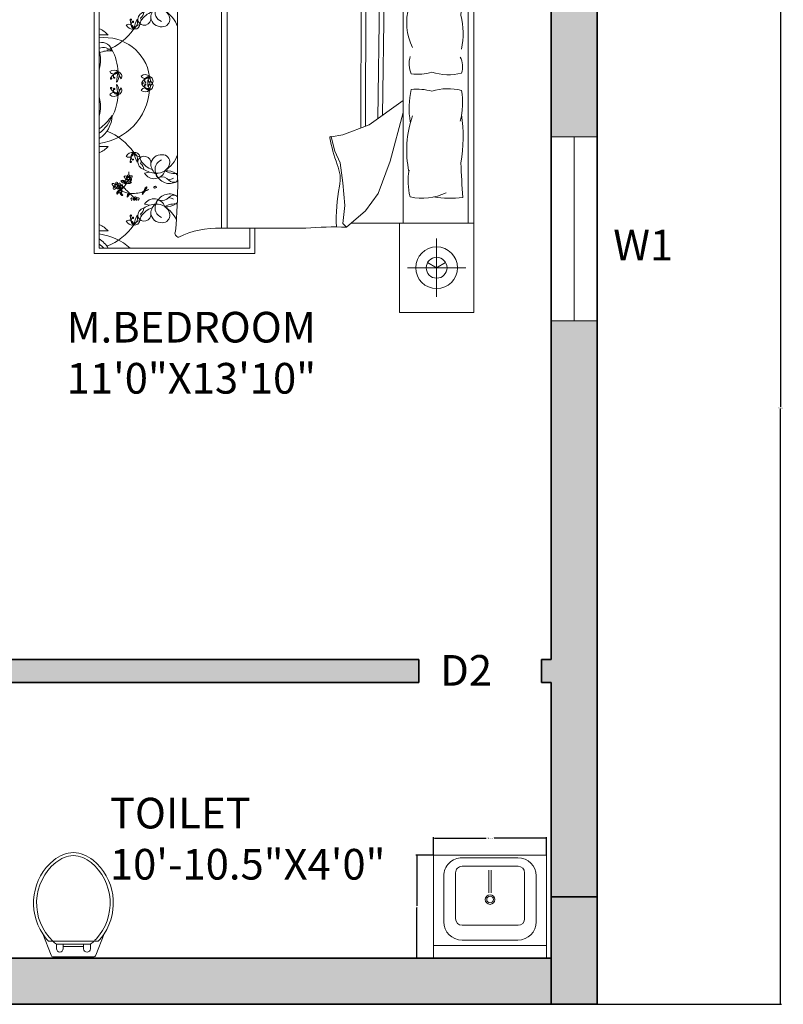
# Model space of a CAD drawing. Units: inches. Extents: x -9 to 505, y -680 to 48.
# Tile 5 of 17: x 356 to 505, y -680 to -487. Entities that reach past the tile are written whole.
import ezdxf

# ---------------------------------------------------------------- set-up
doc = ezdxf.new("R2010")
doc.units = ezdxf.units.IN
doc.header["$MEASUREMENT"] = 0
for name, color, linetype, lineweight in [('A-ANNO-DIMS', 2, 'Continuous', 18), ('A-ANNO-TEXT', 7, 'Continuous', 18), ('A-AREA-IDEN', 7, 'Continuous', 18), ('A-FLOR-FIXT', 9, 'Continuous', 18), ('A-FURN', 8, 'Continuous', 18), ('A-GLAZ', 4, 'Continuous', 18), ('A-WALL', 7, 'Continuous', 35), ('A-WALL-PATT', 251, 'Continuous', 13), ('S-CONC', 7, 'Continuous', 35), ('S-CONC-PATT', 18, 'Continuous', 13), ('WC-Detail_dwgmodels.com', 251, 'Continuous', 13), ('WC-Outline_dwgmodels.com', 250, 'Continuous', 18)]:
    doc.layers.add(name, color=color, linetype=linetype, lineweight=lineweight)
doc.styles.get("Standard").update_dxf_attribs({"font": 'arial.ttf'})
doc.dimstyles.get("Standard").update_dxf_attribs({"dimtxt": 0.18, "dimasz": 0.18, "dimexe": 0.18, "dimexo": 0.0625, "dimgap": 0.09, "dimtad": 0, "dimtih": 1, "dimtoh": 1, "dimdec": 0, "dimzin": 0, "dimdsep": 46, "dimlunit": 3, "dimtxsty": 'Standard', "dimcen": 0.09, "dimadec": 0, "dimazin": 0, "dimtfac": 1, "dimtdec": 0, "dimtofl": 0, "dimtmove": 0, "dimatfit": 3, "dimfxl": 1, "dimtolj": 1, "dimtzin": 0, "dimarcsym": 0})

# ---------------------------------------------------------------- blocks, each defined once
blk = doc.blocks.new('М14 600х655')
for p, q in [((-655, 600), (-655, 0)), ((-655, 600), (-655, 0)), ((-655, 0), (-655, 600)), ((0, 600), (-655, 600)), ((0, 0), (0, 600)), ((0, 525), (-655, 525)), ((-165.1, 494.1), (-489.9, 494.1)), ((-165.4, 408.4), (-490.2, 408.4)), ((-595.8, 388.1), (-595.8, 121.3)), ((-528.4, 370.1), (-528.4, 103.3)), ((-127.2, 103.3), (-127.2, 370.1)), ((-59.2, 121.3), (-59.2, 388.1)), ((-333.5, 87.1), (-333.5, 219.6)), ((-321.5, 87.1), (-321.5, 219.6)), ((-490.2, 65.1), (-165.4, 65.1)), ((-655, 0), (-655, 0)), ((-655, 0), (-655, 0)), ((-655, 0), (0, 0)), ((-655, 0), (0, 0)), ((-489.9, 15.4), (-165.1, 15.4))]:
    blk.add_line(p, q)
for radius in [27.6, 19.3]:
    blk.add_circle((-327.5, 258.9), radius)
for centre, radius, start, end in [((-489.9, 388.1), 105.9, 90, 180), ((-165.1, 388.1), 105.9, 0, 90), ((-490.2, 370.1), 38.2, 90, 180), ((-165.4, 370.1), 38.2, 0, 90), ((-489.9, 121.3), 105.9, 180, 270), ((-165.1, 121.3), 105.9, 270, 0), ((-490.2, 103.3), 38.2, 180, 270), ((-165.4, 103.3), 38.2, 270, 0)]:
    blk.add_arc(centre, radius, start, end)
blk = doc.blocks.new('BED-DOUBLE-WITH-NIGHTSTANDS')
for p, q in [((74.3, 0), (74.3, 87.37)), ((67.02, 72.93), (67.02, 84.34)), ((61.31, 78.63), (72.73, 78.63)), ((0, 75.23), (0, 11.53)), ((31.47, 75.23), (0, 75.23)), ((31.47, 70.38), (31.47, 75.23)), ((1.01, 74.22), (30.46, 74.22)), ((1.01, 12.54), (1.01, 74.22)), ((30.46, 74.22), (30.46, 70.37)), ((24.93, 70.38), (24.93, 16.47)), ((26.02, 70.29), (26.02, 16.47)), ((52.32, 69.59), (52.18, 36.06)), ((53.22, 69.58), (53.09, 36.41)), ((55.97, 69.63), (55.52, 37.9)), ((56.87, 69.66), (56.43, 38.56)), ((60.5, 17.47), (60.5, 69.9)), ((73.18, 69.9), (73.18, 17.47)), ((9.87, 65.61), (10.86, 65.8)), ((16.35, 61.42), (16.35, 25.95)), ((9.87, 59.5), (10.86, 59.31)), ((60.5, 41.48), (53.83, 36.69)), ((57.9, 29.61), (60.5, 39.14)), ((53.83, 36.69), (48.7, 34.74)), ((48.7, 34.74), (46.4, 34.39)), ((46.4, 34.39), (47.11, 31.56)), ((47.11, 31.56), (48.17, 29.26)), ((48.17, 29.26), (48.7, 25.36)), ((55.6, 23.24), (57.9, 29.61)), ((9.87, 27.26), (10.86, 27.45)), ((48.7, 25.36), (49.06, 20.94)), ((53.12, 19.88), (55.6, 23.24)), ((9.87, 21.15), (10.86, 20.96)), ((49.06, 20.94), (48.7, 17.4)), ((49.41, 16.69), (53.12, 19.88)), ((48.7, 17.4), (49.41, 16.69)), ((74.3, 17.47), (50.32, 17.47)), ((30.46, 16.47), (30.46, 12.54)), ((31.47, 11.53), (31.47, 16.47)), ((67.02, 14.45), (67.02, 3.03)), ((30.46, 12.54), (1.01, 12.54)), ((0, 11.53), (31.47, 11.53)), ((61.31, 8.74), (72.73, 8.74))]:
    blk.add_line(p, q)
for points in [[(74.3, 69.9), (59.74, 69.9), (59.74, 87.37), (74.3, 87.37)], [(67.02, 78.63), (65.26, 77.62)], [(67.02, 78.63), (68.79, 77.62)], [(59.74, 17.47), (59.74, 0), (74.3, 0)], [(67.02, 8.74), (65.26, 9.76)], [(67.02, 8.74), (68.79, 9.76)]]:
    blk.add_lwpolyline(points)
for points in [[(26.71, 70.27, -0.056112), (21.91, 70.9, -0.095341), (17.28, 72.13)], [(72.13, 64.88, 0.074897), (66.42, 64.77, -0.472817)], [(66.1, 47.01, 0.14099), (71.92, 46.83, 0.235245)], [(66.1, 43.28, -0.14099), (71.92, 43.45, -0.235245)], [(72.13, 22.49, -0.074897), (66.42, 22.6, 0.472817)], [(41.41, 16.51, -0.001242), (24.83, 16.47, 0.127202), (16.57, 14.72)]]:
    blk.add_lwpolyline(points, format="xyb")
for centre, radius in [((67.02, 78.63), 4.08), ((67.02, 78.63), 2.04), ((4.36, 62.02), 0.223), ((6.7, 60.56), 0.223), ((6.7, 26.2), 0.223), ((4.36, 24.75), 0.223), ((67.02, 8.74), 4.08), ((67.02, 8.74), 2.04)]:
    blk.add_circle(centre, radius)
for centre, radius, start, end in [((-2.05, 76.99), 5.56, 303.4617, 330.1116), ((-3.09, 78.99), 6.93, 306.3036, 316.4814), ((-0.53, 82.71), 11.41, 277.745, 311.8856), ((-1.65, 63.19), 11.41, 34.3865, 68.5908), ((16.83, 71.47), 0.796, 56.1736, 203.4781), ((-0.77, 73.87), 4.64, 292.5547, 318.9546), ((1.73, 86.58), 15.79, 267.4081, 273.6519), ((7.49, 68.4), 1.27, 77.7115, 159.0387), ((6.81, 69.66), 0.953, 238.4633, 358.2869), ((9.93, 67.74), 2.89, 138.8402, 177.9352), ((8.2, 68.81), 0.933, 117.6827, 223.7762), ((7.99, 68.72), 0.946, 2.9516, 103.728), ((15.55, 71.37), 7.98, 192.5173, 207.1824), ((6.71, 68.17), 1.8, 345.4653, 54.2343), ((9.43, 70.65), 1.95, 211.3827, 255.2969), ((-68.63, 64.1), 85.02, 358.1965, 4.7598), ((44.11, 274.32), 204.79, 265.1265, 270.8855), ((49.82, 226.53), 156.99, 269.0718, 273.9), ((7.19, 67.84), 0.142, 177.9352, 11.4834), ((7.26, 67.85), 0.0688, 11.4834, 127.9409), ((7.66, 68.26), 0.0744, 223.7729, 159.7333), ((9.8, 67.61), 1.31, 350.264, 160.8688), ((10.19, 67.92), 1.64, 175.969, 254.3045), ((8.38, 67.88), 0.804, 333.9755, 53.2681), ((8.02, 66.16), 1.74, 6.1662, 51.5825), ((12.69, 70.21), 4.12, 211.2614, 251.7045), ((13.16, 67.13), 2.09, 84.9449, 172.8857), ((13.96, 66.31), 2.03, 111.5819, 201.4221), ((12.28, 68.18), 2.63, 265.2933, 346.921), ((13.37, 67.73), 1.48, 354.4856, 91.0538), ((10.2, 71.58), 6.61, 303.6671, 336.3547), ((12.35, 70.24), 4.69, 236.2883, 266.5076), ((11.75, 66.69), 2.17, 209.9085, 343.1337), ((13.63, 67.49), 2.54, 182.3591, 234.0401), ((14.13, 62.72), 3.37, 122.7011, 126.3445), ((15.71, 69.16), 3.62, 238.8218, 280.751), ((14.13, 62.72), 3.37, 55.785, 94.7304), ((4.68, 63.45), 0.248, 124.3538, 214.3923), ((5.21, 63.62), 0.673, 176.9701, 248.2913), ((10.01, 67.17), 6.5, 212.6784, 216.3746), ((5.6, 63.28), 0.579, 122.8155, 187.3992), ((5.86, 63.21), 0.673, 109.4799, 177.6828), ((5.5, 63.63), 0.248, 56.8636, 146.9021), ((10.97, 60.13), 6.5, 145.1882, 148.8844), ((8.96, 64.13), 2.46, 178.3264, 187.1302), ((6.3, 63.79), 0.459, 11.3256, 64.4621), ((7.86, 64.45), 1.38, 190.2588, 210.656), ((6.93, 63.89), 0.419, 188.3432, 274.2869), ((7.3, 64.12), 0.732, 210.656, 242.6341), ((7.85, 64.75), 1.4, 218.2101, 226.3071), ((6.82, 63.57), 0.178, 325.7657, 67.4417), ((1.29, 69.52), 8.3, 313.1541, 322.0459), ((7.39, 64.54), 0.171, 142.4737, 265.053), ((7.61, 64.57), 0.367, 127.7621, 169.0403), ((7.42, 64.88), 0.517, 265.053, 338.3618), ((8.1, 64.17), 0.676, 113.4276, 137.6104), ((8.03, 64.87), 0.223, 183.2768, 356.7232), ((8.19, 64.47), 0.364, 139.7889, 227.6792), ((8.07, 64.34), 0.192, 227.6792, 350.3487), ((7.33, 64.48), 0.728, 353.0852, 15.7171), ((7.81, 64.39), 0.46, 350.3487, 43.6538), ((8.66, 64.86), 0.535, 198.7263, 262.5032), ((8.24, 64.61), 0.213, 1.1081, 91.8675), ((8.64, 64.5), 0.172, 255.2356, 54.9248), ((8.37, 64.57), 0.371, 11.5637, 52.6358), ((11.9, 63.61), 2.46, 178.3264, 187.1302), ((9.24, 63.27), 0.459, 11.3256, 64.4621), ((10.8, 63.93), 1.38, 190.2588, 210.656), ((12.67, 65.32), 0.542, 167.3041, 285.1471), ((14.77, 66.35), 2.78, 199.2822, 299.1751), ((13.28, 63.06), 1.79, 41.5653, 105.1471), ((14.26, 66.77), 2.51, 277.436, 299.9149), ((15.59, 65.12), 1.31, 221.5653, 293.8354), ((15.39, 64.67), 1.05, 17.4186, 52.325), ((15.39, 64.67), 1.05, 314.4517, 343.3657), ((73.15, 61.76), 11.71, 165.1039, 191.0369), ((64.13, 53.75), 11.26, 65.1316, 101.7583), ((903.62, 16.72), 832.89, 176.68521, 177.14978), ((3.72, 61.68), 0.171, 142.4737, 265.053), ((3.95, 61.71), 0.367, 61.2196, 169.0403), ((3.75, 62.02), 0.517, 265.053, 338.3618), ((4.19, 62.47), 0.439, 157.4086, 261.4386), ((3.94, 62.48), 0.22, 58.0499, 135.6268), ((4.44, 61.32), 0.676, 113.4276, 137.6104), ((4.17, 62.34), 0.147, 172.906, 277.132), ((3.69, 62.07), 0.702, 14.7558, 58.0499), ((4.52, 61.61), 0.364, 139.7889, 227.6792), ((4.67, 62.26), 0.303, 36.1046, 181.4281), ((3.66, 61.62), 0.728, 353.0852, 15.7171), ((4.14, 61.53), 0.46, 350.3487, 43.6538), ((5.05, 63.41), 0.579, 190.3057, 287.1958), ((4.49, 62.5), 0.306, 270.0645, 331.1507), ((4.75, 62.43), 0.35, 221.8413, 265.7877), ((4.99, 62.01), 0.535, 198.7263, 262.5032), ((4.57, 61.76), 0.213, 1.1081, 91.8675), ((4.75, 62.29), 0.218, 263.7526, 41.7054), ((4.7, 61.71), 0.371, 11.5637, 86.365), ((4.99, 63.46), 0.257, 216.3746, 291.7548), ((7.26, 59.85), 3.63, 124.0033, 132.4917), ((4.97, 61.64), 0.172, 255.2356, 54.9248), ((3.53, 59.39), 3.88, 63.7819, 68.2913), ((5.6, 62.38), 0.616, 128.3208, 208.8162), ((5.71, 62.42), 0.737, 207.7043, 254.3516), ((5.16, 63.04), 0.194, 289.3605, 111.7548), ((5.3, 63.04), 0.194, 221.8703, 44.2646), ((6.18, 62.48), 1.01, 157.2305, 229.0635), ((5.84, 62.81), 0.597, 174.4544, 220.6188), ((5.23, 62), 1.01, 270.278, 342.111), ((2.45, 59.48), 4.35, 30.544, 49.818), ((5.62, 63.36), 0.257, 148.8844, 224.2646), ((4.84, 61.96), 0.717, 340.0041, 40.6188), ((7.26, 59.85), 3.63, 94.756, 119.2041), ((14.99, 54.63), 11.94, 132.2412, 142.1744), ((5.71, 62.03), 0.597, 278.7227, 324.8872), ((6.81, 61.72), 0.616, 182.8499, 266.1226), ((6.57, 62.16), 0.597, 231.7607, 277.9252), ((7.04, 62.26), 1.01, 214.5369, 286.3699), ((7.45, 56.25), 7.24, 73.5842, 93.8277), ((9.87, 63.37), 0.419, 188.3432, 274.2869), ((10.24, 63.6), 0.732, 210.656, 242.6341), ((10.79, 64.23), 1.4, 218.2101, 226.3071), ((9.76, 63.05), 0.178, 325.7657, 67.4417), ((10.26, 62.72), 0.419, 147.5332, 233.4768), ((10.63, 62.94), 0.732, 179.1859, 211.164), ((9.92, 62.77), 0.178, 354.3784, 96.0543), ((7.45, 56.25), 7.24, 63.0032, 69.8941), ((11.19, 63.27), 1.38, 211.164, 231.5612), ((11.43, 64.4), 2.46, 234.6898, 243.4936), ((11.45, 63.13), 1.4, 195.5129, 203.6099), ((9.87, 62.21), 0.459, 357.3579, 50.4944), ((11.84, 62.3), 0.168, 12.7051, 190.4384), ((11.95, 62.32), 0.274, 190.4384, 10.4136), ((4.41, 61.49), 0.192, 227.6792, 350.3487), ((5.91, 60.73), 0.717, 98.7227, 159.3375), ((5.55, 61.65), 0.737, 244.9899, 291.6373), ((5.61, 61.55), 0.616, 290.5253, 358.5375), ((6.07, 60.22), 0.171, 142.4737, 265.053), ((6.29, 60.26), 0.367, 61.2196, 169.0403), ((6.1, 60.57), 0.517, 265.053, 338.3618), ((6.53, 61.01), 0.439, 157.4086, 261.4386), ((6.29, 61.03), 0.22, 58.0499, 135.6268), ((6.78, 59.86), 0.676, 113.4276, 137.6104), ((6.52, 60.89), 0.147, 172.906, 277.132), ((6.03, 60.62), 0.702, 14.7558, 58.0499), ((2.45, 59.48), 4.35, 23.0501, 23.8477), ((6.87, 60.16), 0.364, 139.7889, 227.6792), ((6.75, 60.03), 0.192, 227.6792, 350.3487), ((6.75, 60.86), 0.717, 37.3105, 97.9252), ((7.01, 60.81), 0.303, 36.1046, 181.4281), ((6.01, 60.16), 0.728, 353.0852, 15.7171), ((6.83, 61.84), 0.737, 265.0106, 311.658), ((2.45, 59.48), 4.35, 357.1071, 4.7585), ((6.49, 60.07), 0.46, 350.3487, 43.6538), ((7.34, 60.55), 0.535, 198.7263, 262.5032), ((6.84, 61.04), 0.306, 270.0645, 331.1507), ((7.1, 60.97), 0.35, 221.8413, 265.7877), ((6.91, 60.3), 0.213, 1.1081, 91.8675), ((7.1, 60.84), 0.218, 263.7526, 41.7054), ((7.05, 60.25), 0.371, 11.5637, 86.365), ((7.31, 60.19), 0.172, 255.2356, 54.9248), ((11.75, 58.42), 2.17, 16.8663, 150.0915), ((12.67, 59.79), 0.542, 74.8529, 192.6959), ((14.77, 58.76), 2.78, 60.8249, 160.7178), ((13.28, 62.05), 1.79, 254.8529, 318.4347), ((14.26, 58.33), 2.51, 60.0851, 82.564), ((15.59, 59.99), 1.31, 66.1646, 138.4347), ((15.39, 60.44), 1.05, 307.675, 336.7144), ((15.39, 60.44), 1.05, 23.2856, 45.5483), ((72.29, 56.71), 11.12, 163.8254, 206.1239), ((10.19, 57.19), 1.64, 105.6955, 184.031), ((8.02, 58.95), 1.74, 308.4175, 353.8338), ((12.69, 54.9), 4.12, 108.2955, 148.7386), ((12.35, 54.86), 4.69, 93.4924, 123.7117), ((13.63, 57.62), 2.54, 125.9599, 177.6409), ((13.96, 58.8), 2.03, 158.5779, 248.4181), ((12.28, 56.93), 2.63, 13.079, 94.7067), ((14.13, 62.39), 3.37, 233.6555, 237.2989), ((15.71, 55.95), 3.62, 79.7133, 121.1782), ((14.13, 62.39), 3.37, 265.2696, 304.215), ((10.2, 53.53), 6.61, 21.4941, 56.3329), ((56.84, 54.51), 15.36, 348.8159, 13.6573), ((6.81, 55.44), 0.953, 1.7131, 121.5367), ((7.49, 56.71), 1.27, 200.9613, 282.2885), ((7.19, 57.27), 0.142, 348.5166, 182.0648), ((9.93, 57.37), 2.89, 182.0648, 221.1598), ((7.26, 57.26), 0.0688, 232.0591, 348.5166), ((8.2, 56.3), 0.933, 136.2238, 242.3173), ((7.61, 56.86), 0.123, 200.2817, 136.2238), ((6.71, 56.94), 1.8, 305.7657, 14.5347), ((15.55, 53.74), 7.98, 152.8176, 167.4827), ((7.99, 56.39), 0.946, 256.272, 357.0484), ((9.43, 54.46), 1.95, 104.7031, 148.6173), ((9.8, 57.5), 1.31, 199.1312, 9.736), ((8.38, 57.23), 0.804, 306.7319, 26.0245), ((13.16, 57.98), 2.09, 187.1143, 275.0551), ((13.37, 57.38), 1.48, 268.9462, 5.5144), ((-0.77, 51.23), 4.64, 41.0454, 67.4453), ((1.73, 38.53), 15.79, 86.3481, 92.5919), ((-1.65, 61.92), 11.41, 291.4092, 325.6135), ((2.11, 44.94), 8.83, 8.1803, 97.1364), ((1.49, 50.77), 2.05, 10.9261, 103.6102), ((1.78, 49.23), 2.59, 48.0951, 107.1391), ((-4.99, 49.37), 6.27, 343.5431, 17.0202), ((2.92, 46.08), 5.11, 83.3805, 111.883), ((-6.64, 46.18), 11.41, 4.4623, 27.4146), ((66.26, 48.62), 4.63, 161.4593, 204.9817), ((67.77, 48.03), 4.32, 343.8974, 26.6563), ((-8.22, 46.89), 9.28, 4.3787, 5.6357), ((-14.58, 42), 16.58, 19.7217, 19.9028), ((3.89, 46.13), 1.27, 47.7873, 129.1145), ((3.93, 47.57), 0.953, 208.5391, 328.3627), ((5.67, 44.34), 2.89, 108.9159, 148.011), ((4.7, 46.14), 0.933, 87.7585, 193.852), ((12.35, 44.68), 7.98, 162.593, 177.2582), ((3.09, 46.33), 1.8, 315.5411, 24.3101), ((6.69, 47.12), 1.95, 181.4585, 225.3727), ((4.47, 46.16), 0.946, 333.0274, 73.8037), ((10, 45.26), 1.27, 47.7873, 129.1145), ((63.18, 57.31), 10.71, 264.0129, 285.8293), ((3.35, 45.79), 0.142, 148.011, 341.5592), ((3.42, 45.77), 0.0688, 341.5592, 98.0167), ((3.96, 45.93), 0.0744, 193.9791, 129.8091), ((12.35, 44.99), 7.98, 182.7418, 197.407), ((3.09, 43.35), 1.8, 335.6899, 44.4589), ((10.04, 46.7), 0.953, 208.5391, 328.3627), ((9.46, 44.92), 0.142, 148.011, 341.5592), ((9.46, 44.75), 0.142, 18.4408, 211.989), ((11.79, 43.47), 2.89, 108.9159, 148.011), ((11.79, 46.21), 2.89, 211.989, 251.0841), ((9.53, 44.9), 0.0688, 341.5592, 98.0167), ((9.53, 44.78), 0.0688, 261.9833, 18.4408), ((10.81, 45.26), 0.933, 87.7585, 193.852), ((10.81, 44.41), 0.933, 166.148, 272.2415), ((10.03, 44.6), 0.123, 230.0755, 166.148), ((10.07, 45.06), 0.0744, 193.9791, 129.8091), ((9.21, 45.45), 1.8, 315.5411, 24.3101), ((18.47, 43.81), 7.98, 162.593, 177.2582), ((9.21, 44.22), 1.8, 335.6899, 44.4589), ((18.47, 45.87), 7.98, 182.7418, 197.407), ((10.59, 45.29), 0.946, 333.0274, 73.8037), ((12.8, 46.25), 1.95, 181.4585, 225.3727), ((10.59, 44.39), 0.946, 286.1963, 26.9726), ((12.8, 43.43), 1.95, 134.6273, 178.5415), ((-0.53, 44.37), 11.41, 277.745, 355.5377), ((3.93, 42.1), 0.953, 31.6373, 151.4609), ((3.89, 43.54), 1.27, 230.8855, 312.2127), ((3.35, 43.88), 0.142, 18.4408, 211.989), ((5.67, 45.33), 2.89, 211.989, 251.0841), ((3.42, 43.9), 0.0688, 261.9833, 18.4408), ((-6.64, 43.49), 11.41, 332.5854, 355.5377), ((4.7, 43.54), 0.933, 166.148, 272.2415), ((3.92, 43.73), 0.123, 230.0755, 166.148), ((6.69, 42.55), 1.95, 134.6273, 178.5415), ((4.47, 43.51), 0.946, 286.1963, 26.9726), ((10.04, 42.98), 0.953, 31.6373, 151.4609), ((10, 44.41), 1.27, 230.8855, 312.2127), ((77.04, 40), 15.41, 166.3762, 190.1383), ((63.18, 32.98), 10.71, 74.1707, 95.9871), ((56.52, 41.16), 15.57, 346.04, 8.4751), ((-4.99, 40.3), 6.27, 342.9798, 16.4569), ((-8.22, 42.79), 9.28, 354.3643, 355.6213), ((-14.58, 47.67), 16.58, 340.0972, 340.2783), ((40.51, 34.46), 31.69, 350.503, 7.7804), ((-2.05, 38.64), 5.56, 303.4617, 358.728), ((-5.04, 44.28), 10.31, 305.947, 325.9877), ((-3.09, 40.64), 6.93, 306.3036, 342.1496), ((81.47, 31.77), 20.31, 160.7385, 191.9603), ((-1.65, 24.85), 11.41, 34.3865, 68.5908), ((46.33, 34.19), 0.211, 70.2464, 181.1377), ((79.42, 40.46), 33.88, 190.6617, 199.8806), ((1.73, 48.24), 15.79, 267.4081, 273.6519), ((-0.77, 35.53), 4.64, 292.5547, 318.9546), ((7.49, 30.05), 1.27, 77.7115, 159.0387), ((6.81, 31.32), 0.953, 238.4633, 358.2869), ((9.93, 29.39), 2.89, 138.8402, 177.9352), ((8.2, 30.46), 0.933, 117.6827, 223.7762), ((7.99, 30.37), 0.946, 2.9516, 103.728), ((9.43, 32.3), 1.95, 211.3827, 255.2969), ((6.71, 29.83), 1.8, 345.4653, 54.2343), ((15.55, 33.02), 7.98, 192.5173, 207.1824), ((13.16, 28.78), 2.09, 84.9449, 172.8857), ((13.37, 29.38), 1.48, 354.4856, 91.0538), ((7.19, 29.49), 0.142, 177.9352, 11.4834), ((7.26, 29.5), 0.0688, 11.4834, 127.9409), ((7.66, 29.92), 0.0744, 223.7729, 159.7333), ((9.8, 29.26), 1.31, 350.264, 160.8688), ((10.19, 29.57), 1.64, 175.969, 254.3045), ((8.38, 29.53), 0.804, 333.9755, 53.2681), ((8.02, 27.81), 1.74, 6.1662, 51.5825), ((12.69, 31.86), 4.12, 211.2614, 251.7045), ((13.63, 29.14), 2.54, 182.3591, 234.0401), ((13.96, 27.96), 2.03, 111.5819, 201.4221), ((12.28, 29.84), 2.63, 265.2933, 346.921), ((10.2, 33.24), 6.61, 303.6671, 338.5059), ((41.05, 26.07), 7.11, 348.6608, 23.7384), ((903.62, 70.65), 832.89, 182.85022, 183.31479), ((2.45, 27.28), 4.35, 355.2415, 2.8929), ((12.35, 31.9), 4.69, 236.2883, 266.5076), ((11.75, 28.34), 2.17, 209.9085, 343.1337), ((12.67, 26.97), 0.542, 167.3041, 285.1471), ((14.13, 24.37), 3.37, 122.7011, 126.3445), ((14.77, 28.01), 2.78, 199.2822, 299.1751), ((15.71, 30.81), 3.62, 238.8218, 280.2867), ((14.13, 24.37), 3.37, 55.785, 94.7304), ((15.39, 26.33), 1.05, 23.2856, 52.325), ((73.15, 25.61), 11.71, 168.9631, 194.8961), ((3.72, 25.08), 0.171, 94.947, 217.5263), ((3.75, 24.74), 0.517, 21.6382, 94.947), ((4.52, 25.15), 0.364, 132.3208, 220.2111), ((4.41, 25.28), 0.192, 9.6513, 132.3208), ((3.66, 25.14), 0.728, 344.2829, 6.9148), ((4.14, 25.23), 0.46, 316.3462, 9.6513), ((4.99, 24.76), 0.535, 97.4968, 161.2737), ((4.97, 25.12), 0.172, 305.0752, 104.7644), ((5.71, 24.34), 0.737, 105.6484, 152.2957), ((6.18, 24.28), 1.01, 130.9365, 202.7695), ((5.55, 25.11), 0.737, 68.3627, 115.0101), ((5.23, 24.76), 1.01, 17.889, 89.722), ((5.91, 26.03), 0.717, 200.6625, 261.2773), ((2.45, 27.28), 4.35, 310.182, 329.456), ((4.84, 24.8), 0.717, 319.3812, 19.9959), ((5.71, 24.73), 0.597, 35.1128, 81.2773), ((5.61, 25.22), 0.616, 1.4625, 69.4747), ((6.07, 26.54), 0.171, 94.947, 217.5263), ((6.29, 26.51), 0.367, 190.9597, 298.7804), ((6.1, 26.19), 0.517, 21.6382, 94.947), ((6.53, 25.75), 0.439, 98.5614, 202.5914), ((6.29, 25.74), 0.22, 224.3732, 301.9501), ((6.81, 25.04), 0.616, 93.8774, 177.1501), ((7.04, 24.5), 1.01, 73.6301, 145.4631), ((6.57, 24.61), 0.597, 82.0748, 128.2393), ((6.78, 26.9), 0.676, 222.3896, 246.5724), ((6.52, 25.87), 0.147, 82.868, 187.094), ((6.03, 26.14), 0.702, 301.9501, 345.2442), ((2.45, 27.28), 4.35, 336.1523, 336.9499), ((6.87, 26.61), 0.364, 132.3208, 220.2111), ((6.75, 26.73), 0.192, 9.6513, 132.3208), ((6.75, 25.91), 0.717, 262.0748, 322.6895), ((6.01, 26.6), 0.728, 344.2829, 6.9148), ((7.01, 25.96), 0.303, 178.5719, 323.8954), ((6.83, 24.92), 0.737, 48.342, 94.9894), ((6.49, 26.69), 0.46, 316.3462, 9.6513), ((7.34, 26.21), 0.535, 97.4968, 161.2737), ((7.1, 25.79), 0.35, 94.2123, 138.1587), ((6.84, 25.72), 0.306, 28.8493, 89.9355), ((6.91, 26.46), 0.213, 268.1325, 358.8919), ((7.05, 26.51), 0.371, 273.635, 348.4363), ((7.1, 25.92), 0.218, 318.2946, 96.2474), ((7.31, 26.58), 0.172, 305.0752, 104.7644), ((13.28, 24.72), 1.79, 41.5653, 105.1471), ((14.26, 28.43), 2.51, 277.436, 299.9149), ((15.59, 26.77), 1.31, 221.5653, 293.8354), ((-74.6, 24.91), 90.96, 354.3113, 0.6567), ((15.39, 26.33), 1.05, 314.4517, 336.771), ((3.95, 25.05), 0.367, 190.9597, 298.7804), ((4.19, 24.29), 0.439, 98.5614, 202.5914), ((3.94, 24.28), 0.22, 224.3732, 301.9501), ((4.44, 25.45), 0.676, 222.3896, 246.5724), ((4.17, 24.42), 0.147, 82.868, 187.094), ((3.69, 24.69), 0.702, 301.9501, 345.2442), ((4.67, 24.5), 0.303, 178.5719, 323.8954), ((4.68, 23.31), 0.248, 145.6077, 235.6462), ((5.05, 23.35), 0.579, 72.8042, 169.6943), ((4.75, 24.34), 0.35, 94.2123, 138.1587), ((4.49, 24.26), 0.306, 28.8493, 89.9355), ((5.21, 23.14), 0.673, 111.7087, 183.0299), ((10.01, 19.6), 6.5, 143.6254, 147.3216), ((4.57, 25.01), 0.213, 268.1325, 358.8919), ((4.7, 25.05), 0.371, 273.635, 348.4363), ((4.75, 24.47), 0.218, 318.2946, 96.2474), ((4.99, 23.3), 0.257, 68.2452, 143.6254), ((7.26, 26.91), 3.63, 227.5083, 235.9967), ((3.53, 27.37), 3.88, 291.7087, 296.2181), ((5.6, 24.39), 0.616, 151.1838, 231.6792), ((5.6, 23.48), 0.579, 172.6008, 237.1845), ((5.16, 23.72), 0.194, 248.2452, 70.6395), ((5.3, 23.72), 0.194, 315.7354, 138.1297), ((5.86, 23.55), 0.673, 182.3172, 250.5201), ((5.84, 23.95), 0.597, 139.3812, 185.5456), ((5.62, 23.4), 0.257, 135.7354, 211.1156), ((10.97, 26.63), 6.5, 211.1156, 214.8118), ((7.26, 26.91), 3.63, 240.7959, 265.244), ((14.99, 32.13), 11.94, 217.8256, 227.7588), ((6.93, 22.88), 0.419, 85.7131, 171.6568), ((7.3, 22.64), 0.732, 117.3659, 149.344), ((6.82, 23.19), 0.178, 292.5583, 34.2343), ((7.45, 30.51), 7.24, 266.1723, 286.4158), ((1.29, 17.24), 8.3, 37.9541, 46.8459), ((10.8, 22.83), 1.38, 149.344, 169.7412), ((11.9, 23.15), 2.46, 172.8698, 181.6736), ((9.24, 23.49), 0.459, 295.5379, 348.6744), ((9.87, 23.4), 0.419, 85.7131, 171.6568), ((10.24, 23.16), 0.732, 117.3659, 149.344), ((10.79, 22.54), 1.4, 133.6929, 141.7899), ((9.76, 23.71), 0.178, 292.5583, 34.2343), ((10.26, 24.04), 0.419, 126.5232, 212.4668), ((10.63, 23.83), 0.732, 148.836, 180.8141), ((9.92, 23.99), 0.178, 263.9457, 5.6216), ((7.45, 30.51), 7.24, 290.1059, 296.9968), ((11.19, 23.49), 1.38, 128.4388, 148.836), ((11.43, 22.37), 2.46, 116.5064, 125.3102), ((11.45, 23.63), 1.4, 156.3901, 164.4871), ((9.87, 24.55), 0.459, 309.5056, 2.6421), ((11.95, 24.44), 0.274, 349.5864, 169.5616), ((11.84, 24.46), 0.168, 169.5616, 347.2949), ((14.77, 20.41), 2.78, 60.8249, 160.7178), ((80.35, 18.19), 32.98, 168.6608, 182.5481), ((64.13, 33.62), 11.26, 258.2417, 294.8684), ((5.5, 23.13), 0.248, 213.0979, 303.1364), ((7.86, 22.31), 1.38, 149.344, 169.7412), ((8.96, 22.63), 2.46, 172.8698, 181.6736), ((6.3, 22.97), 0.459, 295.5379, 348.6744), ((7.85, 22.01), 1.4, 133.6929, 141.7899), ((7.39, 22.23), 0.171, 94.947, 217.5263), ((7.61, 22.19), 0.367, 190.9597, 232.2379), ((7.42, 21.88), 0.517, 21.6382, 94.947), ((8.1, 22.59), 0.676, 222.3896, 246.5724), ((8.03, 21.89), 0.223, 3.2768, 176.7232), ((8.19, 22.29), 0.364, 132.3208, 220.2111), ((8.07, 22.42), 0.192, 9.6513, 132.3208), ((7.33, 22.29), 0.728, 344.2829, 6.9148), ((7.81, 22.37), 0.46, 316.3462, 9.6513), ((8.66, 21.9), 0.535, 97.4968, 161.2737), ((8.24, 22.15), 0.213, 268.1325, 358.8919), ((8.64, 22.26), 0.172, 305.0752, 104.7644), ((8.37, 22.2), 0.371, 307.3642, 348.4363), ((12.35, 16.52), 4.69, 93.4924, 123.7117), ((11.75, 20.07), 2.17, 16.8663, 150.0915), ((13.63, 19.27), 2.54, 125.9599, 177.6409), ((13.96, 20.46), 2.03, 158.5779, 248.4181), ((12.28, 18.58), 2.63, 13.079, 94.7067), ((12.67, 21.45), 0.542, 74.8529, 192.6959), ((14.13, 24.04), 3.37, 233.6555, 237.2989), ((13.28, 23.7), 1.79, 254.8529, 318.4347), ((15.71, 17.61), 3.62, 80.8446, 121.1782), ((14.13, 24.04), 3.37, 265.2696, 304.215), ((14.26, 19.99), 2.51, 60.0851, 82.564), ((15.59, 21.64), 1.31, 66.1646, 138.4347), ((15.39, 22.09), 1.05, 307.675, 329.9707), ((15.39, 22.09), 1.05, 26.442, 45.5483), ((10.19, 18.84), 1.64, 105.6955, 184.031), ((9.8, 19.16), 1.31, 199.1312, 9.736), ((8.02, 20.61), 1.74, 308.4175, 353.8338), ((12.69, 16.56), 4.12, 108.2955, 148.7386), ((13.16, 19.64), 2.09, 187.1143, 275.0551), ((10.2, 15.18), 6.61, 26.7003, 56.3329), ((6.81, 17.1), 0.953, 1.7131, 121.5367), ((7.49, 18.36), 1.27, 200.9613, 282.2885), ((7.19, 18.93), 0.142, 348.5166, 182.0648), ((9.93, 19.03), 2.89, 182.0648, 221.1598), ((7.26, 18.91), 0.0688, 232.0591, 348.5166), ((8.2, 17.95), 0.933, 136.2238, 242.3173), ((7.61, 18.51), 0.123, 200.2817, 136.2238), ((15.55, 15.4), 7.98, 152.8176, 167.4827), ((6.71, 18.59), 1.8, 305.7657, 14.5347), ((9.43, 16.11), 1.95, 104.7031, 148.6173), ((7.99, 18.05), 0.946, 256.272, 357.0484), ((8.38, 18.89), 0.804, 306.7319, 26.0245), ((13.37, 19.03), 1.48, 268.9462, 5.5144), ((-0.77, 12.89), 4.64, 41.0454, 67.4453), ((1.73, 0.18), 15.79, 86.3481, 92.5919), ((-1.65, 23.57), 11.41, 291.4092, 325.6135), ((16.63, 15.52), 0.806, 152.6588, 266.02), ((47.24, -63.42), 80.14, 88.447, 94.1706), ((-0.53, 4.05), 11.41, 48.1144, 82.255), ((-2.05, 9.77), 5.56, 29.8884, 56.5383), ((-3.09, 7.77), 6.93, 43.5186, 53.6964)]:
    blk.add_arc(centre, radius, start, end)
blk = doc.blocks.new('WIN-36')
for p, q in [((0, 36), (0, 0)), ((9, 36), (0, 36)), ((4.5, 36), (4.5, 2.23)), ((9, 0), (9, 36)), ((4.5, 2.23), (4.5, 0)), ((0, 0), (9, 0))]:
    blk.add_line(p, q)
blk = doc.blocks.new('*D34')
at = {"layer": 'A-ANNO-DIMS', "color": 0, "lineweight": -2, "transparency": 16777216}
for p, q in [((436.76, -650.23), (436.76, -646.8)), ((436.94, -646.98), (446.98, -646.98)), ((458.64, -646.98), (448.6, -646.98)), ((458.82, -650.23), (458.82, -646.8))]:
    blk.add_line(p, q, dxfattribs=at)
at = {"layer": 'A-ANNO-DIMS', "color": 0, "transparency": 16777216}
for points in [[(436.94, -646.95), (436.94, -647.01), (436.76, -646.98)], [(458.64, -646.95), (458.64, -647.01), (458.82, -646.98)]]:
    blk.add_solid(points, dxfattribs=at)
at = {"layer": 'Defpoints', "color": 0, "transparency": 16777216}
for p in [(436.76, -646.98), (436.76, -650.29), (458.82, -650.29)]:
    blk.add_point(p, dxfattribs=at)
at = {"layer": 'A-ANNO-DIMS', "color": 0, "transparency": 16777216, "insert": (447.79, -646.98), "char_height": 0.18, "attachment_point": 5}
blk.add_mtext('\\A1;BASIN 1\'-10"', dxfattribs=at)
blk = doc.blocks.new('*D35')
at = {"layer": 'A-ANNO-DIMS', "color": 0, "lineweight": -2, "transparency": 16777216}
for p, q in [((436.7, -650.29), (433.27, -650.29)), ((433.45, -650.47), (433.45, -660.21)), ((433.45, -670.32), (433.45, -660.58)), ((436.7, -670.5), (433.27, -670.5))]:
    blk.add_line(p, q, dxfattribs=at)
at = {"layer": 'A-ANNO-DIMS', "color": 0, "transparency": 16777216}
for points in [[(433.42, -650.47), (433.48, -650.47), (433.45, -650.29)], [(433.42, -670.32), (433.48, -670.32), (433.45, -670.5)]]:
    blk.add_solid(points, dxfattribs=at)
at = {"layer": 'Defpoints', "color": 0, "transparency": 16777216}
for p in [(436.76, -650.29), (433.45, -670.5), (436.76, -670.5)]:
    blk.add_point(p, dxfattribs=at)
at = {"layer": 'A-ANNO-DIMS', "color": 0, "transparency": 16777216, "insert": (433.45, -660.4), "char_height": 0.18, "attachment_point": 5}
blk.add_mtext('\\A1;1\'-8"', dxfattribs=at)
blk = doc.blocks.new('*D48')
at = {"layer": 'A-ANNO-DIMS', "color": 0, "lineweight": -2, "transparency": 16777216}
for p, q in [((459.83, -446), (504.82, -446)), ((504.64, -446.18), (504.64, -562.57)), ((504.64, -679.32), (504.64, -562.93)), ((468.83, -679.5), (504.82, -679.5))]:
    blk.add_line(p, q, dxfattribs=at)
at = {"layer": 'A-ANNO-DIMS', "color": 0, "transparency": 16777216}
for points in [[(504.61, -446.18), (504.67, -446.18), (504.64, -446)], [(504.61, -679.32), (504.67, -679.32), (504.64, -679.5)]]:
    blk.add_solid(points, dxfattribs=at)
at = {"layer": 'Defpoints', "color": 0, "transparency": 16777216}
for p in [(459.76, -446), (468.76, -679.5), (504.64, -679.5)]:
    blk.add_point(p, dxfattribs=at)
at = {"layer": 'A-ANNO-DIMS', "color": 0, "transparency": 16777216, "insert": (504.64, -562.75), "char_height": 0.18, "attachment_point": 5}
blk.add_mtext('\\A1;19\'-5 1/2"', dxfattribs=at)

msp = doc.modelspace()

# ---------------------------------------------------------------- hatches: boundary and pattern name
at = {"layer": 'A-WALL-PATT'}
h = msp.add_hatch(color=256, dxfattribs=at)
h.dxf.hatch_style = 1
h.paths.add_polyline_path([(101.64, 11.5), (48.26, 11.5), (48.26, 2.5), (72.26, 2.5), (72.26, -21.25), (81.26, -21.25), (81.26, 2.5), (101.64, 2.5)])
h.paths.add_polyline_path([(36.26, 2.5), (27.26, 2.5), (27.26, -6.92), (36.26, -6.92)])
h.paths.add_polyline_path([(81.26, -57.25), (72.26, -57.25), (72.26, -75.5), (81.26, -75.5)])
h.paths.add_polyline_path([(162.76, 11.5), (137.64, 11.5), (137.64, 2.5), (162.76, 2.5)])
h.paths.add_polyline_path([(179.26, 2.5), (174.76, 2.5), (174.76, -75.5), (179.26, -75.5), (179.26, -54.5), (229.51, -54.5), (229.51, -45.5), (179.26, -45.5)])
h.paths.add_polyline_path([(382.26, -45.5), (332.26, -45.5), (332.26, 2.5), (327.76, 2.5), (327.76, -45.5), (277.51, -45.5), (277.51, -54.5), (327.76, -54.5), (327.76, -111.5), (332.26, -111.5), (332.26, -54.5), (382.26, -54.5)])
h.paths.add_polyline_path([(332.26, -128), (327.76, -128), (327.76, -207), (332.26, -207)])
h.paths.add_polyline_path([(124.76, -111.5), (36.26, -111.5), (36.26, -116), (120.26, -116), (120.26, -168.5), (179.26, -168.5), (179.26, -164), (124.76, -164)])
h.paths.add_polyline_path([(96.26, -164), (36.26, -164), (36.26, -152), (27.26, -152), (27.26, -208.88), (36.26, -208.88), (36.26, -168.5), (96.26, -168.5)])
h.paths.add_polyline_path([(36.26, -244.88), (27.26, -244.88), (27.26, -287), (36.26, -287)])
h.paths.add_polyline_path([(179.26, -204.5), (174.76, -204.5), (174.76, -287), (179.26, -287)])
h.paths.add_polyline_path([(257.26, -296), (248.26, -296), (248.26, -446), (269.26, -446), (269.26, -437), (257.26, -437)])
h.paths.add_polyline_path([(90.26, -296), (81.26, -296), (81.26, -348.67), (90.26, -348.67)])
h.paths.add_polyline_path([(90.26, -384.67), (81.26, -384.67), (81.26, -416), (90.26, -416)])
h.paths.add_polyline_path([(170.26, -452), (36.26, -452), (36.26, -456.5), (165.76, -456.5), (165.76, -504.5), (165.13, -504.5), (165.13, -509), (170.26, -509)])
h.paths.add_polyline_path([(141.76, -504.5), (36.26, -504.5), (36.26, -492.5), (27.26, -492.5), (27.26, -565.96), (36.26, -565.96), (36.26, -509), (141.76, -509)])
h.paths.add_polyline_path([(36.26, -601.96), (27.26, -601.96), (27.26, -658.5), (36.26, -658.5)])
h.paths.add_polyline_path([(170.26, -670.5), (170.26, -634.5), (222.76, -634.5), (222.76, -625.5), (165.76, -625.5), (165.76, -670.5), (36.26, -670.5), (36.26, -679.5), (170.26, -679.5)])
h.paths.add_polyline_path([(332.26, -616.5), (433.89, -616.5), (433.89, -612), (332.26, -612), (332.26, -610.56), (327.76, -610.56), (327.76, -625.5), (270.76, -625.5), (270.76, -634.5), (327.76, -634.5), (327.76, -658.5), (332.26, -658.5)])
h.paths.add_polyline_path([(459.76, -670.5), (336.76, -670.5), (336.76, -679.5), (459.76, -679.5)])
h.paths.add_polyline_path([(468.76, -545.74), (459.76, -545.74), (459.76, -612), (457.89, -612), (457.89, -616.5), (459.76, -616.5), (459.76, -658.5), (468.76, -658.5)])
h.paths.add_polyline_path([(332.26, -446), (327.76, -446), (327.76, -574.56), (332.26, -574.56)])
h.paths.add_polyline_path([(327.76, -437), (305.26, -437), (305.26, -446), (327.76, -446)])
h.paths.add_polyline_path([(459.76, -437), (348.76, -437), (348.76, -446), (459.76, -446)])
h.paths.add_polyline_path([(468.76, -458), (459.76, -458), (459.76, -509.74), (468.76, -509.74)])
h.paths.add_polyline_path([(468.76, -365), (459.76, -365), (459.76, -437), (468.76, -437)])
h.paths.add_polyline_path([(468.76, -299.6), (459.76, -299.6), (459.76, -344), (468.76, -344)])
h.paths.add_polyline_path([(468.76, -184.74), (459.76, -184.74), (459.76, -231), (401.26, -231), (401.26, -235.5), (459.76, -235.5), (459.76, -275.6), (468.76, -275.6)])
h.paths.add_polyline_path([(390.76, -356), (342.76, -356), (342.76, -365), (390.76, -365)])
h.paths.add_polyline_path([(459.76, -356), (405.76, -356), (405.76, -365), (459.76, -365)])
h.paths.add_polyline_path([(405.76, -296), (396.76, -296), (396.76, -356), (405.76, -356)])
h.paths.add_polyline_path([(336.76, -296), (327.76, -296), (327.76, -356), (336.76, -356)])
h.paths.add_polyline_path([(468.76, -9.5), (459.76, -9.5), (459.76, -45.5), (418.26, -45.5), (418.26, -54.5), (468.76, -54.5)])
h.paths.add_polyline_path([(468.76, -54.5), (459.76, -54.5), (459.76, -111.5), (468.76, -111.5)])
h.paths.add_polyline_path([(468.76, -128), (459.76, -128), (459.76, -148.74), (468.76, -148.74)])
at = {"layer": 'S-CONC-PATT'}
h = msp.add_hatch(color=256, dxfattribs=at)
h.dxf.hatch_style = 1
h.paths.add_polyline_path([(336.76, -658.5), (327.76, -658.5), (327.76, -679.5), (336.76, -679.5), (336.76, -670.5)])
h.paths.add_polyline_path([(468.76, -658.5), (459.76, -658.5), (459.76, -679.5), (468.76, -679.5)])
h.paths.add_polyline_path([(36.26, -658.5), (27.26, -658.5), (27.26, -679.5), (36.26, -679.5)])

# ---------------------------------------------------------------- linework, layer by layer
at = {"layer": 'A-WALL'}
for p, q in [((468.76, 11.5), (468.76, -679.5)), ((459.76, -235.5), (459.76, -612)), ((332.26, -612), (433.89, -612)), ((433.89, -616.5), (433.89, -612)), ((457.89, -612), (457.89, -616.5)), ((457.89, -612), (459.76, -612)), ((332.26, -616.5), (433.89, -616.5)), ((457.89, -616.5), (459.76, -616.5)), ((459.76, -616.5), (459.76, -679.5)), ((336.76, -670.5), (459.76, -670.5)), ((27.26, -679.5), (468.76, -679.5))]:
    msp.add_line(p, q, dxfattribs=at)
at = {"layer": 'S-CONC'}
msp.add_line((459.76, -658.5), (468.76, -658.5), dxfattribs=at)
at = {"layer": 'WC-Detail_dwgmodels.com'}
for p, q in [((362.25, -667.15), (361.39, -667.15)), ((371.15, -667.15), (370.29, -667.15))]:
    msp.add_line(p, q, dxfattribs=at)
for points in [[(361.39, -667.15, -0.040937), (360.29, -665.74, -0.163732)], [(371.15, -667.15, 0.040937), (372.26, -665.74, 0.163732)], [(362.96, -667.76, -0.022712), (362.25, -667.15, -0.162618)], [(366.27, -667.76), (362.96, -667.76, -0.476108)], [(362.96, -667.76), (362.96, -668.62, 1), (364.26, -668.62), (364.26, -668.18)], [(366.27, -667.76), (369.59, -667.76, 0.022712)], [(369.59, -667.76), (369.59, -668.62, -1), (368.28, -668.62), (368.28, -668.18)], [(369.59, -667.76, 0.022712), (370.29, -667.15, 0.162618)]]:
    msp.add_lwpolyline(points, format="xyb", dxfattribs=at)
for points in [[(364.26, -668.18), (364.26, -667.76)], [(364.26, -668.18), (368.28, -668.18)], [(368.28, -668.18), (368.28, -667.76)]]:
    msp.add_lwpolyline(points, dxfattribs=at)
at = {"layer": 'WC-Outline_dwgmodels.com'}
for p in [(362.25, -667.15), (370.29, -667.15)]:
    msp.add_line(p, (366.27, -667.15), dxfattribs=at)
for points in [[(360.29, -665.74, -0.383919), (362.43, -651.28, -0.163732), (366.27, -649.8, -0.359733)], [(362.25, -667.15, -0.448546), (362.82, -651.75, -0.162618), (366.27, -650.41, -0.470877)], [(372.26, -665.74, 0.383919), (370.11, -651.28, 0.163732), (366.27, -649.8, 0.359733)], [(370.7, -666.73, 0.431639), (369.72, -651.75, 0.162618), (366.27, -650.41, 0.470877)], [(366.27, -670.24), (362.37, -670.24, -0.31031), (361.89, -669.91), (360.29, -665.74, -0.209071)], [(366.27, -670.24), (370.17, -670.24, 0.31031), (370.65, -669.91), (372.26, -665.74, 0.209071)], [(370.29, -667.15, 0.014165), (370.7, -666.73, 0.162618)]]:
    msp.add_lwpolyline(points, format="xyb", dxfattribs=at)

# ---------------------------------------------------------------- block references
at = {"layer": 'A-FLOR-FIXT', "xscale": 0.0336812458408458, "yscale": 0.0336812458408458, "zscale": 0.0336812458408458, "rotation": 180}
msp.add_blockref('М14 600х655', (436.76, -650.29), dxfattribs=at)
at = {"layer": 'A-FURN'}
msp.add_blockref('BED-DOUBLE-WITH-NIGHTSTANDS', (370.32, -544.1), dxfattribs=at)
at = {"layer": 'A-GLAZ'}
msp.add_blockref('WIN-36', (459.76, -545.74), dxfattribs=at)

# ---------------------------------------------------------------- texts
at = {"layer": 'A-ANNO-TEXT', "char_height": 6, "attachment_point": 1}
for s, insert in [('W1', (471.9, -527.92)), ('D2', (438.02, -611.15))]:
    msp.add_mtext(s, dxfattribs=dict(at, insert=insert))
at = {"layer": 'A-AREA-IDEN', "insert": (364.95, -543.99), "char_height": 6, "attachment_point": 1}
msp.add_mtext('M.BEDROOM\\P11\'0"X13\'10"', dxfattribs=at)
at = {"layer": 'A-AREA-IDEN', "insert": (373.41, -639.09), "char_height": 6, "attachment_point": 1}
msp.add_mtext_dynamic_manual_height_columns('TOILET\\P10\'-10.5"X4\'0"', width=0.6495, gutter_width=1, heights=[0], dxfattribs=at)

# ---------------------------------------------------------------- dimensions: what is measured, and where the dimension line sits
at = {"layer": 'A-ANNO-DIMS'}
for base, p1, p2, angle, picture, middle in [((504.64, -679.5), (459.76, -446), (468.76, -679.5), 90, '*D48', (504.64, -562.75)), ((433.45, -670.5), (436.76, -650.29), (436.76, -670.5), 270, '*D35', (433.45, -660.4))]:
    dim = msp.add_linear_dim(base=base, p1=p1, p2=p2, angle=angle, dimstyle='Standard', override={"dimdec": 1, "dimlfac": 1, "dimrnd": 0, "dimzin": 1, "dimdsep": 46, "dimlunit": 4, "dimfrac": 2}, dxfattribs=at)
    dim.commit()
    dim.dimension.update_dxf_attribs({"geometry": picture, "text_midpoint": middle})
dim = msp.add_linear_dim(base=(436.76, -646.98), p1=(458.82, -650.29), p2=(436.76, -650.29), angle=180, text='BASIN <>', dimstyle='Standard', override={"dimdec": 1, "dimlfac": 1, "dimrnd": 0, "dimzin": 1, "dimdsep": 46, "dimlunit": 4, "dimfrac": 2}, dxfattribs=at)
dim.commit()
dim.dimension.update_dxf_attribs({"geometry": '*D34', "text_midpoint": (447.79, -646.98)})

doc.saveas('drawing.dxf')
